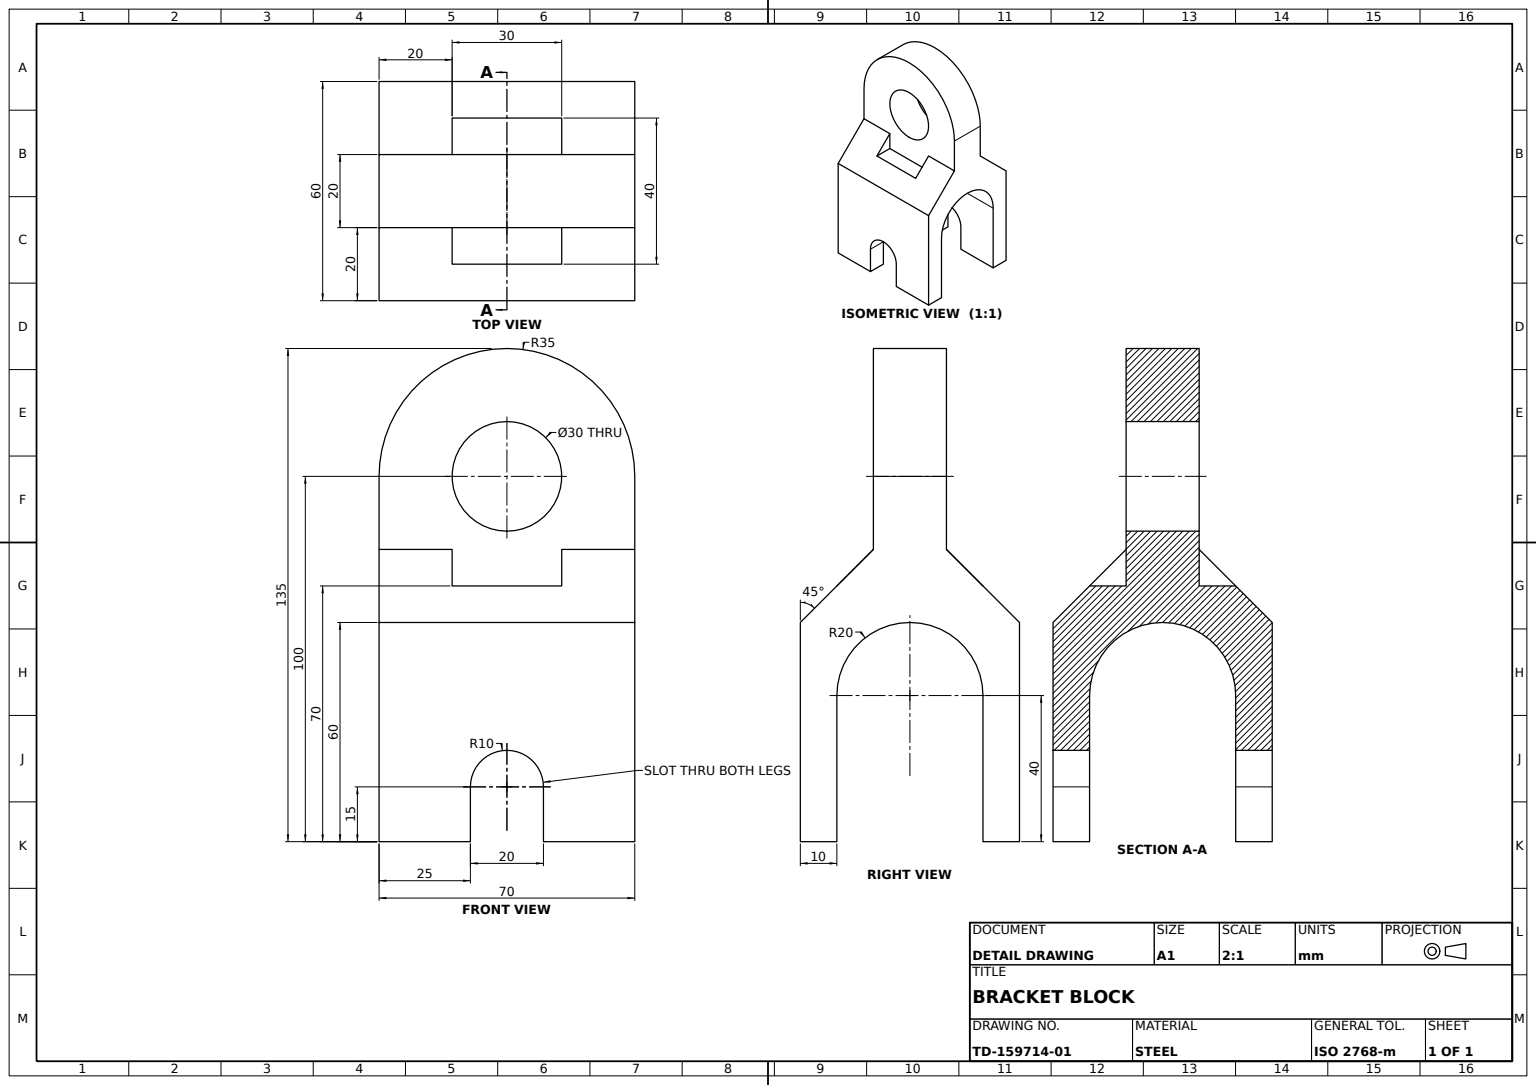
from build123d import *

# Parameters (mm, degrees)
ARCHED_BASE_BLOCK_DEPTH = 35
HINGE_EAR_DEPTH         = 20
HINGE_BORE_DEPTH        = 92.923881554
HINGE_BORE_DEPTH_BACK   = 92.923881554
HINGE_BORE_SKETCH_R     = 15
EAR_START               = 20
EAR_ROOT_NOTCH_SKETCH_W = 30
EAR_ROOT_NOTCH_SKETCH_H = 10
EAR_ROOT_NOTCH_DEPTH    = 10


with BuildPart() as part:
    # Arched Base Profile Sketch → Arched Base Block (new, symmetric)
    with BuildSketch(Plane(origin=(0, 0, 0), x_dir=(0, 0, -1), z_dir=(1, 0, 0))):
        with BuildLine():
            Line((-30, 0), (-10, 20))
            Line((-10, 20), (-10, 40))
            Line((-10, 40), (10, 40))
            Line((10, 40), (10, 20))
            Line((10, 20), (30, 0))
            Line((30, 0), (30, -60))
            Line((30, -60), (20, -60))
            Line((20, -60), (20, -20))
            ThreePointArc((20, -20), (0, 0), (-20, -20))
            Line((-20, -20), (-20, -60))
            Line((-20, -60), (-30, -60))
            Line((-30, -60), (-30, 0))
        make_face()
    extrude(amount=ARCHED_BASE_BLOCK_DEPTH, both=True)

    # Hinge Ear Sketch → Hinge Ear (add)
    with BuildSketch(Plane(origin=(0, 0, -10), x_dir=(-1, 0, 0), z_dir=(0, 0, -1))):
        with BuildLine():
            Line((-35, 40), (35, 40))
            ThreePointArc((35, 40), (0, 75), (-35, 40))
        make_face()
    extrude(amount=-HINGE_EAR_DEPTH)

    # Hinge Bore Sketch → Hinge Bore (cut, two sides: drawn at the far end of the back side and taken through both)
    with BuildSketch(Plane(origin=(0, 0, -10), x_dir=(-1, 0, 0), z_dir=(0, 0, -1)).offset(-HINGE_BORE_DEPTH_BACK)):
        with Locations(Location((0, 40, 0), (0, 0, 90))):
            Circle(HINGE_BORE_SKETCH_R)
        with BuildLine():
            Line((-10, -45), (-10, -60))
            Line((-10, -60), (10, -60))
            Line((10, -60), (10, -45))
            ThreePointArc((10, -45), (0, -35), (-10, -45))
        make_face()
    extrude(amount=HINGE_BORE_DEPTH + HINGE_BORE_DEPTH_BACK, mode=Mode.SUBTRACT)

    # Ear Root Notch Sketch → Ear Root Notch (cut)
    with BuildSketch(Plane(origin=(0, 0, 0), x_dir=(1, 0, 0), z_dir=(0, 1, 0)).offset(EAR_START)):
        with Locations((0, 15)):
            Rectangle(EAR_ROOT_NOTCH_SKETCH_W, EAR_ROOT_NOTCH_SKETCH_H)
    ear_root_notch = extrude(amount=-EAR_ROOT_NOTCH_DEPTH, mode=Mode.SUBTRACT)

    # Ear Root Notch Mirror: Ear Root Notch across plane
    add(ear_root_notch.mirror(Plane.XY), mode=Mode.SUBTRACT)


solid = part.part
